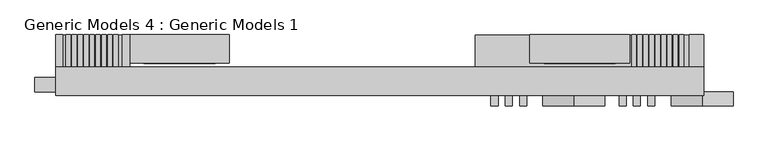
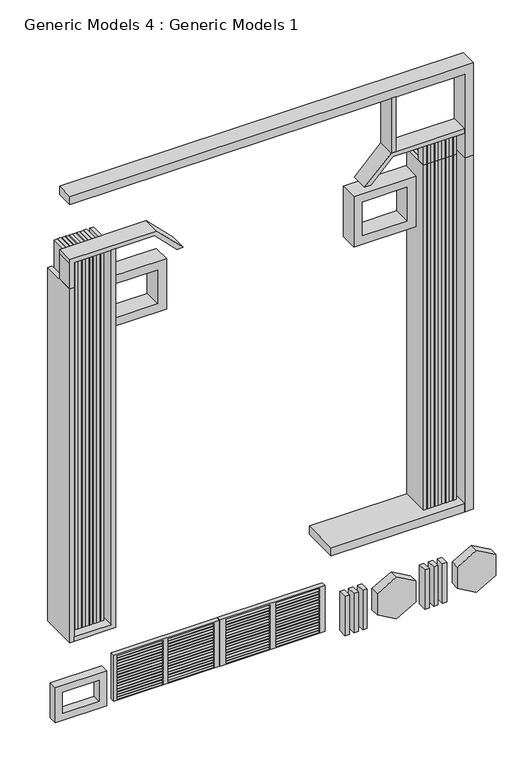
"""IFC4 building model written with IfcOpenShell, lengths in millimetres: proxy geometry, Generic Models 4 : Generic Models 1."""

from ifc_helpers import new_model, si_unit, frame, origin, place, context, project, spatial, polyline, outline, extrude, source, transform, mapped, element, save


def generic_models_4_generic_models_1_75103227(model_context):
    return source(origin(), model_context, "Body", "SweptSolid", [
        extrude(outline(polyline([(1820.8669612, -11572.940066), (1668.4669612, -11572.940066), (1668.4669612, -11268.140066), (1820.8669612, -11268.140066), (1820.8669612, -11572.940066)])), frame((0.0, 0.0, 188.9137514), z_axis=(0.0, 0.0, 1.0), x_axis=(1.0, 0.0, 0.0)), (0.0, 0.0, 1.0), 1422.4),
        extrude(outline(polyline([(2125.6669612, -11572.940066), (1973.2669612, -11572.940066), (1973.2669612, -11268.140066), (2125.6669612, -11268.140066), (2125.6669612, -11572.940066)])), frame((0.0, 0.0, 188.9137514), z_axis=(0.0, 0.0, 1.0), x_axis=(1.0, 0.0, 0.0)), (0.0, 0.0, 1.0), 1422.4),
        extrude(outline(polyline([(2430.4669612, -11572.940066), (2278.0669612, -11572.940066), (2278.0669612, -11268.140066), (2430.4669612, -11268.140066), (2430.4669612, -11572.940066)])), frame((0.0, 0.0, 188.9137514), z_axis=(0.0, 0.0, 1.0), x_axis=(1.0, 0.0, 0.0)), (0.0, 0.0, 1.0), 1422.4),
        extrude(outline(polyline([(1319.1930949, 4094.8824571), (1700.1930949, 3434.9710994), (1319.1930949, 2775.0597417), (557.1930949, 2775.0597417), (176.1930949, 3434.9710994), (557.1930949, 4094.8824571), (1319.1930949, 4094.8824571)])), frame((0.0, -11572.940066, 0.0), z_axis=(0.0, 1.0, 0.0), x_axis=(0.0, 0.0, 1.0)), (0.0, 0.0, 1.0), 304.8),
        extrude(outline(polyline([(4555.5166213, -11572.940066), (4403.1166213, -11572.940066), (4403.1166213, -11268.140066), (4555.5166213, -11268.140066), (4555.5166213, -11572.940066)])), frame((0.0, 0.0, 188.9137514), z_axis=(0.0, 0.0, 1.0), x_axis=(1.0, 0.0, 0.0)), (0.0, 0.0, 1.0), 1422.4),
        extrude(outline(polyline([(4860.3166213, -11572.940066), (4707.9166213, -11572.940066), (4707.9166213, -11268.140066), (4860.3166213, -11268.140066), (4860.3166213, -11572.940066)])), frame((0.0, 0.0, 188.9137514), z_axis=(0.0, 0.0, 1.0), x_axis=(1.0, 0.0, 0.0)), (0.0, 0.0, 1.0), 1422.4),
        extrude(outline(polyline([(5165.1166213, -11572.940066), (5012.7166213, -11572.940066), (5012.7166213, -11268.140066), (5165.1166213, -11268.140066), (5165.1166213, -11572.940066)])), frame((0.0, 0.0, 188.9137514), z_axis=(0.0, 0.0, 1.0), x_axis=(1.0, 0.0, 0.0)), (0.0, 0.0, 1.0), 1422.4),
        extrude(outline(polyline([(1319.1930949, 6838.0824571), (1700.1930949, 6178.1710994), (1319.1930949, 5518.2597417), (557.1930949, 5518.2597417), (176.1930949, 6178.1710994), (557.1930949, 6838.0824571), (1319.1930949, 6838.0824571)])), frame((0.0, -11572.940066, 0.0), z_axis=(0.0, 1.0, 0.0), x_axis=(0.0, 0.0, 1.0)), (0.0, 0.0, 1.0), 304.8),
        extrude(outline(polyline([(1526.1468401, -6316.9793183), (1526.1468401, -8069.5793183), (256.1468401, -8069.5793183), (256.1468401, -6316.9793183), (1526.1468401, -6316.9793183)]), holes=[polyline([(1272.1468401, -6570.9793183), (510.1468401, -6570.9793183), (510.1468401, -7815.5793183), (1272.1468401, -7815.5793183), (1272.1468401, -6570.9793183)])]), frame((0.0, -11268.140066, 0.0), z_axis=(0.0, 1.0, 0.0), x_axis=(0.0, 0.0, 1.0)), (0.0, 0.0, 1.0), 304.8),
        extrude(outline(polyline([(87.200464, 1329.7166213), (1760.22, 1329.7166213), (1760.22, -2250.6971451), (87.200464, -2250.6971451), (87.200464, 1329.7166213)]), holes=[polyline([(1628.5995189, -2050.1814423), (1704.7995189, -2050.1814423), (1704.7995189, -551.5814423), (1628.5995189, -551.5814423), (1628.5995189, -2050.1814423)]), polyline([(1526.9995189, -2050.1814423), (1603.1995189, -2050.1814423), (1603.1995189, -551.5814423), (1526.9995189, -551.5814423), (1526.9995189, -2050.1814423)]), polyline([(1425.3995189, -2050.1814423), (1501.5995189, -2050.1814423), (1501.5995189, -551.5814423), (1425.3995189, -551.5814423), (1425.3995189, -2050.1814423)]), polyline([(1323.7995189, -2050.1814423), (1399.9995189, -2050.1814423), (1399.9995189, -551.5814423), (1323.7995189, -551.5814423), (1323.7995189, -2050.1814423)]), polyline([(1222.1995189, -2050.1814423), (1298.3995189, -2050.1814423), (1298.3995189, -551.5814423), (1222.1995189, -551.5814423), (1222.1995189, -2050.1814423)]), polyline([(1120.5995189, -2050.1814423), (1196.7995189, -2050.1814423), (1196.7995189, -551.5814423), (1120.5995189, -551.5814423), (1120.5995189, -2050.1814423)]), polyline([(1018.9995189, -2050.1814423), (1095.1995189, -2050.1814423), (1095.1995189, -551.5814423), (1018.9995189, -551.5814423), (1018.9995189, -2050.1814423)]), polyline([(917.3995189, -2050.1814423), (993.5995189, -2050.1814423), (993.5995189, -551.5814423), (917.3995189, -551.5814423), (917.3995189, -2050.1814423)]), polyline([(815.7995189, -2050.1814423), (891.9995189, -2050.1814423), (891.9995189, -551.5814423), (815.7995189, -551.5814423), (815.7995189, -2050.1814423)]), polyline([(714.1995189, -2050.1814423), (790.3995189, -2050.1814423), (790.3995189, -551.5814423), (714.1995189, -551.5814423), (714.1995189, -2050.1814423)]), polyline([(612.5995189, -2050.1814423), (688.7995189, -2050.1814423), (688.7995189, -551.5814423), (612.5995189, -551.5814423), (612.5995189, -2050.1814423)]), polyline([(510.9995189, -2050.1814423), (587.1995189, -2050.1814423), (587.1995189, -551.5814423), (510.9995189, -551.5814423), (510.9995189, -2050.1814423)]), polyline([(409.3995189, -2050.1814423), (485.5995189, -2050.1814423), (485.5995189, -551.5814423), (409.3995189, -551.5814423), (409.3995189, -2050.1814423)]), polyline([(307.7995189, -2050.1814423), (383.9995189, -2050.1814423), (383.9995189, -551.5814423), (307.7995189, -551.5814423), (307.7995189, -2050.1814423)]), polyline([(206.1995189, -2050.1814423), (282.3995189, -2050.1814423), (282.3995189, -551.5814423), (206.1995189, -551.5814423), (206.1995189, -2050.1814423)]), polyline([(117.2995189, -2050.1814423), (193.4995189, -2050.1814423), (193.4995189, -551.5814423), (117.2995189, -551.5814423), (117.2995189, -2050.1814423)]), polyline([(1628.5995189, -346.6833787), (1704.7995189, -346.6833787), (1704.7995189, 1151.9166213), (1628.5995189, 1151.9166213), (1628.5995189, -346.6833787)]), polyline([(1526.9995189, -346.6833787), (1603.1995189, -346.6833787), (1603.1995189, 1151.9166213), (1526.9995189, 1151.9166213), (1526.9995189, -346.6833787)]), polyline([(1425.3995189, -346.6833787), (1501.5995189, -346.6833787), (1501.5995189, 1151.9166213), (1425.3995189, 1151.9166213), (1425.3995189, -346.6833787)]), polyline([(1323.7995189, -346.6833787), (1399.9995189, -346.6833787), (1399.9995189, 1151.9166213), (1323.7995189, 1151.9166213), (1323.7995189, -346.6833787)]), polyline([(1222.1995189, -346.6833787), (1298.3995189, -346.6833787), (1298.3995189, 1151.9166213), (1222.1995189, 1151.9166213), (1222.1995189, -346.6833787)]), polyline([(1120.5995189, -346.6833787), (1196.7995189, -346.6833787), (1196.7995189, 1151.9166213), (1120.5995189, 1151.9166213), (1120.5995189, -346.6833787)]), polyline([(1018.9995189, -346.6833787), (1095.1995189, -346.6833787), (1095.1995189, 1151.9166213), (1018.9995189, 1151.9166213), (1018.9995189, -346.6833787)]), polyline([(917.3995189, -346.6833787), (993.5995189, -346.6833787), (993.5995189, 1151.9166213), (917.3995189, 1151.9166213), (917.3995189, -346.6833787)]), polyline([(815.7995189, -346.6833787), (891.9995189, -346.6833787), (891.9995189, 1151.9166213), (815.7995189, 1151.9166213), (815.7995189, -346.6833787)]), polyline([(714.1995189, -346.6833787), (790.3995189, -346.6833787), (790.3995189, 1151.9166213), (714.1995189, 1151.9166213), (714.1995189, -346.6833787)]), polyline([(612.5995189, -346.6833787), (688.7995189, -346.6833787), (688.7995189, 1151.9166213), (612.5995189, 1151.9166213), (612.5995189, -346.6833787)]), polyline([(510.9995189, -346.6833787), (587.1995189, -346.6833787), (587.1995189, 1151.9166213), (510.9995189, 1151.9166213), (510.9995189, -346.6833787)]), polyline([(409.3995189, -346.6833787), (485.5995189, -346.6833787), (485.5995189, 1151.9166213), (409.3995189, 1151.9166213), (409.3995189, -346.6833787)]), polyline([(307.7995189, -346.6833787), (383.9995189, -346.6833787), (383.9995189, 1151.9166213), (307.7995189, 1151.9166213), (307.7995189, -346.6833787)]), polyline([(206.1995189, -346.6833787), (282.3995189, -346.6833787), (282.3995189, 1151.9166213), (206.1995189, 1151.9166213), (206.1995189, -346.6833787)]), polyline([(117.2995189, -346.6833787), (193.4995189, -346.6833787), (193.4995189, 1151.9166213), (117.2995189, 1151.9166213), (117.2995189, -346.6833787)])]), frame((0.0, -10963.340066, 0.0), z_axis=(0.0, 1.0, 0.0), x_axis=(0.0, 0.0, 1.0)), (0.0, 0.0, 1.0), 152.4),
        extrude(outline(polyline([(1760.22, -5896.5833787), (87.200464, -5896.5833787), (87.200464, -2283.4333787), (1760.22, -2283.4333787), (1760.22, -5896.5833787)]), holes=[polyline([(1628.5995189, -5783.9814423), (1704.7995189, -5783.9814423), (1704.7995189, -4209.1814423), (1628.5995189, -4209.1814423), (1628.5995189, -5783.9814423)]), polyline([(1526.9995189, -5783.9814423), (1603.1995189, -5783.9814423), (1603.1995189, -4209.1814423), (1526.9995189, -4209.1814423), (1526.9995189, -5783.9814423)]), polyline([(1425.3995189, -5783.9814423), (1501.5995189, -5783.9814423), (1501.5995189, -4209.1814423), (1425.3995189, -4209.1814423), (1425.3995189, -5783.9814423)]), polyline([(1323.7995189, -5783.9814423), (1399.9995189, -5783.9814423), (1399.9995189, -4209.1814423), (1323.7995189, -4209.1814423), (1323.7995189, -5783.9814423)]), polyline([(1222.1995189, -5783.9814423), (1298.3995189, -5783.9814423), (1298.3995189, -4209.1814423), (1222.1995189, -4209.1814423), (1222.1995189, -5783.9814423)]), polyline([(1120.5995189, -5783.9814423), (1196.7995189, -5783.9814423), (1196.7995189, -4209.1814423), (1120.5995189, -4209.1814423), (1120.5995189, -5783.9814423)]), polyline([(1018.9995189, -5783.9814423), (1095.1995189, -5783.9814423), (1095.1995189, -4209.1814423), (1018.9995189, -4209.1814423), (1018.9995189, -5783.9814423)]), polyline([(917.3995189, -5783.9814423), (993.5995189, -5783.9814423), (993.5995189, -4209.1814423), (917.3995189, -4209.1814423), (917.3995189, -5783.9814423)]), polyline([(815.7995189, -5783.9814423), (891.9995189, -5783.9814423), (891.9995189, -4209.1814423), (815.7995189, -4209.1814423), (815.7995189, -5783.9814423)]), polyline([(714.1995189, -5783.9814423), (790.3995189, -5783.9814423), (790.3995189, -4209.1814423), (714.1995189, -4209.1814423), (714.1995189, -5783.9814423)]), polyline([(612.5995189, -5783.9814423), (688.7995189, -5783.9814423), (688.7995189, -4209.1814423), (612.5995189, -4209.1814423), (612.5995189, -5783.9814423)]), polyline([(510.9995189, -5783.9814423), (587.1995189, -5783.9814423), (587.1995189, -4209.1814423), (510.9995189, -4209.1814423), (510.9995189, -5783.9814423)]), polyline([(409.3995189, -5783.9814423), (485.5995189, -5783.9814423), (485.5995189, -4209.1814423), (409.3995189, -4209.1814423), (409.3995189, -5783.9814423)]), polyline([(307.7995189, -5783.9814423), (383.9995189, -5783.9814423), (383.9995189, -4209.1814423), (307.7995189, -4209.1814423), (307.7995189, -5783.9814423)]), polyline([(206.1995189, -5783.9814423), (282.3995189, -5783.9814423), (282.3995189, -4209.1814423), (206.1995189, -4209.1814423), (206.1995189, -5783.9814423)]), polyline([(117.2995189, -5783.9814423), (193.4995189, -5783.9814423), (193.4995189, -4209.1814423), (117.2995189, -4209.1814423), (117.2995189, -5783.9814423)]), polyline([(1628.5995189, -4031.3814423), (1704.7995189, -4031.3814423), (1704.7995189, -2456.5814423), (1628.5995189, -2456.5814423), (1628.5995189, -4031.3814423)]), polyline([(1526.9995189, -4031.3814423), (1603.1995189, -4031.3814423), (1603.1995189, -2456.5814423), (1526.9995189, -2456.5814423), (1526.9995189, -4031.3814423)]), polyline([(1425.3995189, -4031.3814423), (1501.5995189, -4031.3814423), (1501.5995189, -2456.5814423), (1425.3995189, -2456.5814423), (1425.3995189, -4031.3814423)]), polyline([(1323.7995189, -4031.3814423), (1399.9995189, -4031.3814423), (1399.9995189, -2456.5814423), (1323.7995189, -2456.5814423), (1323.7995189, -4031.3814423)]), polyline([(1222.1995189, -4031.3814423), (1298.3995189, -4031.3814423), (1298.3995189, -2456.5814423), (1222.1995189, -2456.5814423), (1222.1995189, -4031.3814423)]), polyline([(1120.5995189, -4031.3814423), (1196.7995189, -4031.3814423), (1196.7995189, -2456.5814423), (1120.5995189, -2456.5814423), (1120.5995189, -4031.3814423)]), polyline([(1018.9995189, -4031.3814423), (1095.1995189, -4031.3814423), (1095.1995189, -2456.5814423), (1018.9995189, -2456.5814423), (1018.9995189, -4031.3814423)]), polyline([(917.3995189, -4031.3814423), (993.5995189, -4031.3814423), (993.5995189, -2456.5814423), (917.3995189, -2456.5814423), (917.3995189, -4031.3814423)]), polyline([(815.7995189, -4031.3814423), (891.9995189, -4031.3814423), (891.9995189, -2456.5814423), (815.7995189, -2456.5814423), (815.7995189, -4031.3814423)]), polyline([(714.1995189, -4031.3814423), (790.3995189, -4031.3814423), (790.3995189, -2456.5814423), (714.1995189, -2456.5814423), (714.1995189, -4031.3814423)]), polyline([(612.5995189, -4031.3814423), (688.7995189, -4031.3814423), (688.7995189, -2456.5814423), (612.5995189, -2456.5814423), (612.5995189, -4031.3814423)]), polyline([(510.9995189, -4031.3814423), (587.1995189, -4031.3814423), (587.1995189, -2456.5814423), (510.9995189, -2456.5814423), (510.9995189, -4031.3814423)]), polyline([(409.3995189, -4031.3814423), (485.5995189, -4031.3814423), (485.5995189, -2456.5814423), (409.3995189, -2456.5814423), (409.3995189, -4031.3814423)]), polyline([(307.7995189, -4031.3814423), (383.9995189, -4031.3814423), (383.9995189, -2456.5814423), (307.7995189, -2456.5814423), (307.7995189, -4031.3814423)]), polyline([(206.1995189, -4031.3814423), (282.3995189, -4031.3814423), (282.3995189, -2456.5814423), (206.1995189, -2456.5814423), (206.1995189, -4031.3814423)]), polyline([(117.2995189, -4031.3814423), (193.4995189, -4031.3814423), (193.4995189, -2456.5814423), (117.2995189, -2456.5814423), (117.2995189, -4031.3814423)])]), frame((0.0, -10963.340066, 0.0), z_axis=(0.0, 1.0, 0.0), x_axis=(0.0, 0.0, 1.0)), (0.0, 0.0, 1.0), 152.4),
        extrude(outline(polyline([(-6290.2833787, -11039.540066), (-6391.8833787, -11039.540066), (-6391.8833787, -10048.940066), (-6290.2833787, -10048.940066), (-6290.2833787, -11039.540066)])), frame((0.0, 0.0, 3200.4), z_axis=(0.0, 0.0, 1.0), x_axis=(1.0, 0.0, 0.0)), (0.0, 0.0, 1.0), 13563.6),
        extrude(outline(polyline([(-6417.2833787, -11039.540066), (-6518.8833787, -11039.540066), (-6518.8833787, -10048.940066), (-6417.2833787, -10048.940066), (-6417.2833787, -11039.540066)])), frame((0.0, 0.0, 3200.4), z_axis=(0.0, 0.0, 1.0), x_axis=(1.0, 0.0, 0.0)), (0.0, 0.0, 1.0), 13563.6),
        extrude(outline(polyline([(-6544.2833787, -11039.540066), (-6645.8833787, -11039.540066), (-6645.8833787, -10048.940066), (-6544.2833787, -10048.940066), (-6544.2833787, -11039.540066)])), frame((0.0, 0.0, 3200.4), z_axis=(0.0, 0.0, 1.0), x_axis=(1.0, 0.0, 0.0)), (0.0, 0.0, 1.0), 13563.6),
        extrude(outline(polyline([(-6671.2833787, -11039.540066), (-6772.8833787, -11039.540066), (-6772.8833787, -10048.940066), (-6671.2833787, -10048.940066), (-6671.2833787, -11039.540066)])), frame((0.0, 0.0, 3200.4), z_axis=(0.0, 0.0, 1.0), x_axis=(1.0, 0.0, 0.0)), (0.0, 0.0, 1.0), 13563.6),
        extrude(outline(polyline([(-6798.2833787, -11039.540066), (-6899.8833787, -11039.540066), (-6899.8833787, -10048.940066), (-6798.2833787, -10048.940066), (-6798.2833787, -11039.540066)])), frame((0.0, 0.0, 3200.4), z_axis=(0.0, 0.0, 1.0), x_axis=(1.0, 0.0, 0.0)), (0.0, 0.0, 1.0), 13563.6),
        extrude(outline(polyline([(-6925.2833787, -11039.540066), (-7026.8833787, -11039.540066), (-7026.8833787, -10048.940066), (-6925.2833787, -10048.940066), (-6925.2833787, -11039.540066)])), frame((0.0, 0.0, 3200.4), z_axis=(0.0, 0.0, 1.0), x_axis=(1.0, 0.0, 0.0)), (0.0, 0.0, 1.0), 13563.6),
        extrude(outline(polyline([(-7052.2833787, -11039.540066), (-7153.8833787, -11039.540066), (-7153.8833787, -10048.940066), (-7052.2833787, -10048.940066), (-7052.2833787, -11039.540066)])), frame((0.0, 0.0, 3200.4), z_axis=(0.0, 0.0, 1.0), x_axis=(1.0, 0.0, 0.0)), (0.0, 0.0, 1.0), 13563.6),
        extrude(outline(polyline([(-7179.2833787, -11039.540066), (-7280.8833787, -11039.540066), (-7280.8833787, -10048.940066), (-7179.2833787, -10048.940066), (-7179.2833787, -11039.540066)])), frame((0.0, 0.0, 3200.4), z_axis=(0.0, 0.0, 1.0), x_axis=(1.0, 0.0, 0.0)), (0.0, 0.0, 1.0), 13563.6),
        extrude(outline(polyline([(-7306.2833787, -11039.540066), (-7407.8833787, -11039.540066), (-7407.8833787, -10048.940066), (-7306.2833787, -10048.940066), (-7306.2833787, -11039.540066)])), frame((0.0, 0.0, 3200.4), z_axis=(0.0, 0.0, 1.0), x_axis=(1.0, 0.0, 0.0)), (0.0, 0.0, 1.0), 13563.6),
        extrude(outline(polyline([(5787.4166213, -11039.540066), (5685.8166213, -11039.540066), (5685.8166213, -10734.740066), (5787.4166213, -10734.740066), (5787.4166213, -11039.540066)])), frame((0.0, 0.0, 15849.6), z_axis=(0.0, 0.0, 1.0), x_axis=(1.0, 0.0, 0.0)), (0.0, 0.0, 1.0), 914.4),
        extrude(outline(polyline([(5660.4166213, -11039.540066), (5558.8166213, -11039.540066), (5558.8166213, -10734.740066), (5660.4166213, -10734.740066), (5660.4166213, -11039.540066)])), frame((0.0, 0.0, 15849.6), z_axis=(0.0, 0.0, 1.0), x_axis=(1.0, 0.0, 0.0)), (0.0, 0.0, 1.0), 914.4),
        extrude(outline(polyline([(5533.4166213, -11039.540066), (5431.8166213, -11039.540066), (5431.8166213, -10734.740066), (5533.4166213, -10734.740066), (5533.4166213, -11039.540066)])), frame((0.0, 0.0, 15849.6), z_axis=(0.0, 0.0, 1.0), x_axis=(1.0, 0.0, 0.0)), (0.0, 0.0, 1.0), 914.4),
        extrude(outline(polyline([(5406.4166213, -11039.540066), (5304.8166213, -11039.540066), (5304.8166213, -10734.740066), (5406.4166213, -10734.740066), (5406.4166213, -11039.540066)])), frame((0.0, 0.0, 15849.6), z_axis=(0.0, 0.0, 1.0), x_axis=(1.0, 0.0, 0.0)), (0.0, 0.0, 1.0), 914.4),
        extrude(outline(polyline([(5279.4166213, -11039.540066), (5177.8166213, -11039.540066), (5177.8166213, -10734.740066), (5279.4166213, -10734.740066), (5279.4166213, -11039.540066)])), frame((0.0, 0.0, 15849.6), z_axis=(0.0, 0.0, 1.0), x_axis=(1.0, 0.0, 0.0)), (0.0, 0.0, 1.0), 914.4),
        extrude(outline(polyline([(5152.4166213, -11039.540066), (5050.8166213, -11039.540066), (5050.8166213, -10734.740066), (5152.4166213, -10734.740066), (5152.4166213, -11039.540066)])), frame((0.0, 0.0, 15849.6), z_axis=(0.0, 0.0, 1.0), x_axis=(1.0, 0.0, 0.0)), (0.0, 0.0, 1.0), 914.4),
        extrude(outline(polyline([(5025.4166213, -11039.540066), (4923.8166213, -11039.540066), (4923.8166213, -10734.740066), (5025.4166213, -10734.740066), (5025.4166213, -11039.540066)])), frame((0.0, 0.0, 15849.6), z_axis=(0.0, 0.0, 1.0), x_axis=(1.0, 0.0, 0.0)), (0.0, 0.0, 1.0), 914.4),
        extrude(outline(polyline([(4898.4166213, -11039.540066), (4796.8166213, -11039.540066), (4796.8166213, -10734.740066), (4898.4166213, -10734.740066), (4898.4166213, -11039.540066)])), frame((0.0, 0.0, 15849.6), z_axis=(0.0, 0.0, 1.0), x_axis=(1.0, 0.0, 0.0)), (0.0, 0.0, 1.0), 914.4),
        extrude(outline(polyline([(4771.4166213, -11039.540066), (4669.8166213, -11039.540066), (4669.8166213, -10734.740066), (4771.4166213, -10734.740066), (4771.4166213, -11039.540066)])), frame((0.0, 0.0, 15849.6), z_axis=(0.0, 0.0, 1.0), x_axis=(1.0, 0.0, 0.0)), (0.0, 0.0, 1.0), 914.4),
        extrude(outline(polyline([(5787.4166213, -11039.540066), (5685.8166213, -11039.540066), (5685.8166213, -10048.940066), (5787.4166213, -10048.940066), (5787.4166213, -11039.540066)])), frame((0.0, 0.0, 3352.8), z_axis=(0.0, 0.0, 1.0), x_axis=(1.0, 0.0, 0.0)), (0.0, 0.0, 1.0), 12496.8),
        extrude(outline(polyline([(5660.4166213, -11039.540066), (5558.8166213, -11039.540066), (5558.8166213, -10048.940066), (5660.4166213, -10048.940066), (5660.4166213, -11039.540066)])), frame((0.0, 0.0, 3352.8), z_axis=(0.0, 0.0, 1.0), x_axis=(1.0, 0.0, 0.0)), (0.0, 0.0, 1.0), 12496.8),
        extrude(outline(polyline([(5533.4166213, -11039.540066), (5431.8166213, -11039.540066), (5431.8166213, -10048.940066), (5533.4166213, -10048.940066), (5533.4166213, -11039.540066)])), frame((0.0, 0.0, 3352.8), z_axis=(0.0, 0.0, 1.0), x_axis=(1.0, 0.0, 0.0)), (0.0, 0.0, 1.0), 12496.8),
        extrude(outline(polyline([(5406.4166213, -11039.540066), (5304.8166213, -11039.540066), (5304.8166213, -10048.940066), (5406.4166213, -10048.940066), (5406.4166213, -11039.540066)])), frame((0.0, 0.0, 3352.8), z_axis=(0.0, 0.0, 1.0), x_axis=(1.0, 0.0, 0.0)), (0.0, 0.0, 1.0), 12496.8),
        extrude(outline(polyline([(5279.4166213, -11039.540066), (5177.8166213, -11039.540066), (5177.8166213, -10048.940066), (5279.4166213, -10048.940066), (5279.4166213, -11039.540066)])), frame((0.0, 0.0, 3352.8), z_axis=(0.0, 0.0, 1.0), x_axis=(1.0, 0.0, 0.0)), (0.0, 0.0, 1.0), 12496.8),
        extrude(outline(polyline([(5152.4166213, -11039.540066), (5050.8166213, -11039.540066), (5050.8166213, -10048.940066), (5152.4166213, -10048.940066), (5152.4166213, -11039.540066)])), frame((0.0, 0.0, 3352.8), z_axis=(0.0, 0.0, 1.0), x_axis=(1.0, 0.0, 0.0)), (0.0, 0.0, 1.0), 12496.8),
        extrude(outline(polyline([(5025.4166213, -11039.540066), (4923.8166213, -11039.540066), (4923.8166213, -10048.940066), (5025.4166213, -10048.940066), (5025.4166213, -11039.540066)])), frame((0.0, 0.0, 3352.8), z_axis=(0.0, 0.0, 1.0), x_axis=(1.0, 0.0, 0.0)), (0.0, 0.0, 1.0), 12496.8),
        extrude(outline(polyline([(4898.4166213, -11039.540066), (4796.8166213, -11039.540066), (4796.8166213, -10048.940066), (4898.4166213, -10048.940066), (4898.4166213, -11039.540066)])), frame((0.0, 0.0, 3352.8), z_axis=(0.0, 0.0, 1.0), x_axis=(1.0, 0.0, 0.0)), (0.0, 0.0, 1.0), 12496.8),
        extrude(outline(polyline([(4771.4166213, -11039.540066), (4669.8166213, -11039.540066), (4669.8166213, -10048.940066), (4771.4166213, -10048.940066), (4771.4166213, -11039.540066)])), frame((0.0, 0.0, 3352.8), z_axis=(0.0, 0.0, 1.0), x_axis=(1.0, 0.0, 0.0)), (0.0, 0.0, 1.0), 12496.8),
        extrude(outline(polyline([(3539.5166213, -11344.340066), (3387.1166213, -11344.340066), (3387.1166213, -10734.740066), (3539.5166213, -10734.740066), (3539.5166213, -11344.340066)])), frame((0.0, 0.0, 16916.4), z_axis=(0.0, 0.0, 1.0), x_axis=(1.0, 0.0, 0.0)), (0.0, 0.0, 1.0), 1981.2),
        extrude(outline(polyline([(5901.7166213, -11344.340066), (1329.7166213, -11344.340066), (1329.7166213, -10048.940066), (5901.7166213, -10048.940066), (5901.7166213, -11344.340066)])), frame((0.0, 0.0, 3048.0), z_axis=(0.0, 0.0, 1.0), x_axis=(1.0, 0.0, 0.0)), (0.0, 0.0, 1.0), 304.8),
        extrude(outline(polyline([(3200.4, -6048.9833787), (16764.0, -6048.9833787), (16764.0, -6201.3833787), (3200.4, -6201.3833787), (3200.4, -7471.3833787), (3048.0, -7471.3833787), (3048.0, -6048.9833787), (3200.4, -6048.9833787)])), frame((0.0, -11344.340066, 0.0), z_axis=(0.0, 1.0, 0.0), x_axis=(0.0, 0.0, 1.0)), (0.0, 0.0, 1.0), 1295.4),
        extrude(outline(polyline([(-7471.3833787, -11344.340066), (-7623.7833787, -11344.340066), (-7623.7833787, -10048.940066), (-7471.3833787, -10048.940066), (-7471.3833787, -11344.340066)])), frame((0.0, 0.0, 3048.0), z_axis=(0.0, 0.0, 1.0), x_axis=(1.0, 0.0, 0.0)), (0.0, 0.0, 1.0), 12801.6),
        extrude(outline(polyline([(16916.4, 3387.1166213), (16002.0, 2472.7166213), (16002.0, 2688.2427682), (16764.0, 3450.2427682), (16764.0, 5901.7166213), (16916.4, 5901.7166213), (16916.4, 3387.1166213)])), frame((0.0, -11344.340066, 0.0), z_axis=(0.0, 1.0, 0.0), x_axis=(0.0, 0.0, 1.0)), (0.0, 0.0, 1.0), 609.6),
        extrude(outline(polyline([(16916.4, -4651.9833787), (16916.4, -7623.7833787), (16764.0, -7623.7833787), (15849.6, -7623.7833787), (15849.6, -7471.3833787), (16764.0, -7471.3833787), (16764.0, -4715.1095256), (16002.0, -3953.1095256), (16002.0, -3737.5833787), (16916.4, -4651.9833787)])), frame((0.0, -11344.340066, 0.0), z_axis=(0.0, 1.0, 0.0), x_axis=(0.0, 0.0, 1.0)), (0.0, 0.0, 1.0), 609.6),
        extrude(outline(polyline([(6206.5166213, -11344.340066), (5901.7166213, -11344.340066), (5901.7166213, -10048.940066), (6206.5166213, -10048.940066), (6206.5166213, -11344.340066)])), frame((0.0, 0.0, 3048.0), z_axis=(0.0, 0.0, 1.0), x_axis=(1.0, 0.0, 0.0)), (0.0, 0.0, 1.0), 12801.6),
        extrude(outline(polyline([(18897.6, -7623.7833787), (18897.6, 5901.7166213), (15849.6, 5901.7166213), (15849.6, 6206.5166213), (18897.6, 6206.5166213), (19202.4, 6206.5166213), (19202.4, -7623.7833787), (18897.6, -7623.7833787)])), frame((0.0, -11344.340066, 0.0), z_axis=(0.0, 1.0, 0.0), x_axis=(0.0, 0.0, 1.0)), (0.0, 0.0, 1.0), 609.6),
        extrude(outline(polyline([(15240.0, -3915.3833787), (15240.0, -6048.9833787), (13411.2, -6048.9833787), (13411.2, -3915.3833787), (15240.0, -3915.3833787)]), holes=[polyline([(14935.2, -4220.1833787), (13716.0, -4220.1833787), (13716.0, -5744.1833787), (14935.2, -5744.1833787), (14935.2, -4220.1833787)])]), frame((0.0, -10658.540066, 0.0), z_axis=(0.0, 1.0, 0.0), x_axis=(0.0, 0.0, 1.0)), (0.0, 0.0, 1.0), 609.6),
        extrude(outline(polyline([(15240.0, 4631.7166213), (15240.0, 2498.1166213), (13411.2, 2498.1166213), (13411.2, 4631.7166213), (15240.0, 4631.7166213)]), holes=[polyline([(14935.2, 4326.9166213), (13716.0, 4326.9166213), (13716.0, 2802.9166213), (14935.2, 2802.9166213), (14935.2, 4326.9166213)])]), frame((0.0, -10658.540066, 0.0), z_axis=(0.0, 1.0, 0.0), x_axis=(0.0, 0.0, 1.0)), (0.0, 0.0, 1.0), 609.6),
    ])


if __name__ == "__main__":
    model = new_model("IFC4")
    model_context = context("Model", 3, world=origin())
    ifc_project = project(units=[si_unit("LENGTHUNIT", "METRE", prefix="MILLI")], contexts=[model_context])
    site = spatial("IfcSite", under=ifc_project)
    building = spatial("IfcBuilding", under=site)
    placement = place(None, origin())
    generic_models_4_generic_models_1_shape = generic_models_4_generic_models_1_75103227(model_context)
    element("IfcBuildingElementProxy", 1, Name="Generic Models 4 : Generic Models 1", ObjectType="Generic Models 4 : Generic Models 1", at=placement, inside=building, context=model_context, shape_type="MappedRepresentation", body=[
        mapped(generic_models_4_generic_models_1_shape, transform((0.0, 0.0, 0.0), x_axis=(1.0, 0.0, 0.0), y_axis=(0.0, 1.0, 0.0), z_axis=(0.0, 0.0, 1.0))),
    ])
    save(model, "model.ifc")

# Revit data of these elements
# Element 1 (IfcBuildingElementProxy, "Generic Models 4 : Generic Models 1")
#   Materials on its faces: "9\" wall", "grey", "Wood Planks", "coffee brown", "wood 3"
# Materials
#   "9\" wall": class "Generic", colour RGB 216 199 172, transparency 0, Cost = 0
#   "grey": class "Generic", colour RGB 33 34 34, transparency 0, Cost = 0
#   "Wood Planks": class "Wood", colour RGB 193 160 115, transparency 0, Description = "Physical material.", Cost = 0
#   "coffee brown": class "Generic", colour RGB 89 68 56, transparency 0, Cost = 0
#   "wood 3": class "Generic", colour RGB 120 120 120, transparency 0, Cost = 0
